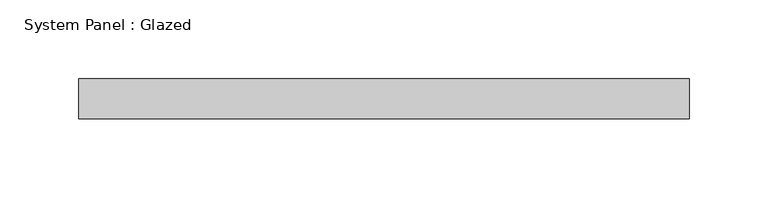
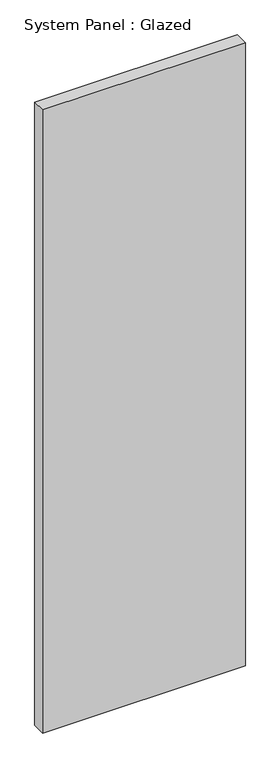
"""IFC4 building model written with IfcOpenShell, lengths in millimetres: plate geometry, System Panel : Glazed."""

from ifc_helpers import new_model, si_unit, origin, origin_with_axes, place, context, project, spatial, polyline, outline, extrude, source, transform, mapped, element, save


def system_panel_glazed_958ccbb4(model_context):
    return source(origin(), model_context, "Body", "SweptSolid", [
        extrude(outline(polyline([(193.675, 19.05), (-193.675, 19.05), (-193.675, 44.45), (193.675, 44.45), (193.675, 19.05)])), origin_with_axes(), (0.0, 0.0, 1.0), 1257.7839289),
    ])


if __name__ == "__main__":
    model = new_model("IFC4")
    model_context = context("Model", 3, world=origin())
    ifc_project = project(units=[si_unit("LENGTHUNIT", "METRE", prefix="MILLI")], contexts=[model_context])
    site = spatial("IfcSite", under=ifc_project)
    building = spatial("IfcBuilding", under=site)
    placement = place(None, origin())
    system_panel_glazed_shape = system_panel_glazed_958ccbb4(model_context)
    element("IfcPlate", 1, ObjectType="System Panel : Glazed", at=placement, inside=building, context=model_context, shape_type="MappedRepresentation", body=[
        mapped(system_panel_glazed_shape, transform((0.0, 0.0, 0.0), x_axis=(1.0, 0.0, 0.0), y_axis=(0.0, 1.0, 0.0), z_axis=(0.0, 0.0, 1.0))),
    ])
    save(model, "model.ifc")

# Revit data of these elements
# Type "System Panel : Glazed"
#   Construction Type Id = "GSP4R"
#   Analytic Construction = "1/8 in Pilkington single glazing"
#   Visual Light Transmittance = 0.9
#   Solar Heat Gain Coefficient = 0.86
#   Heat Transfer Coefficient (U) = 1.18115 BTU/(h·ft²·°F)
#   Define Thermal Properties by = 1
# Element 1 (IfcPlate, "System Panel : Glazed")
#   Materials on its faces: "Glass"
# Materials
#   "Glass": class "Glass", colour RGB 0 128 192, transparency 0.75, Description = "Soda Lime Glass", Cost = 0
